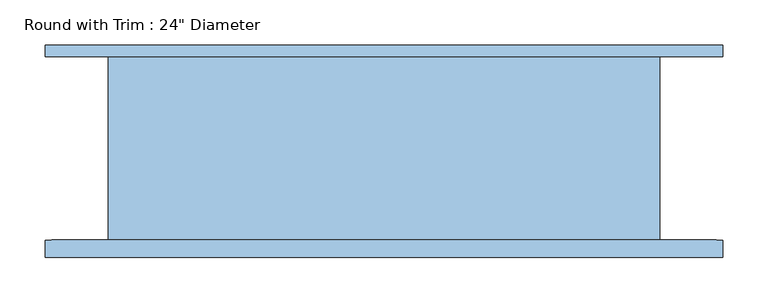
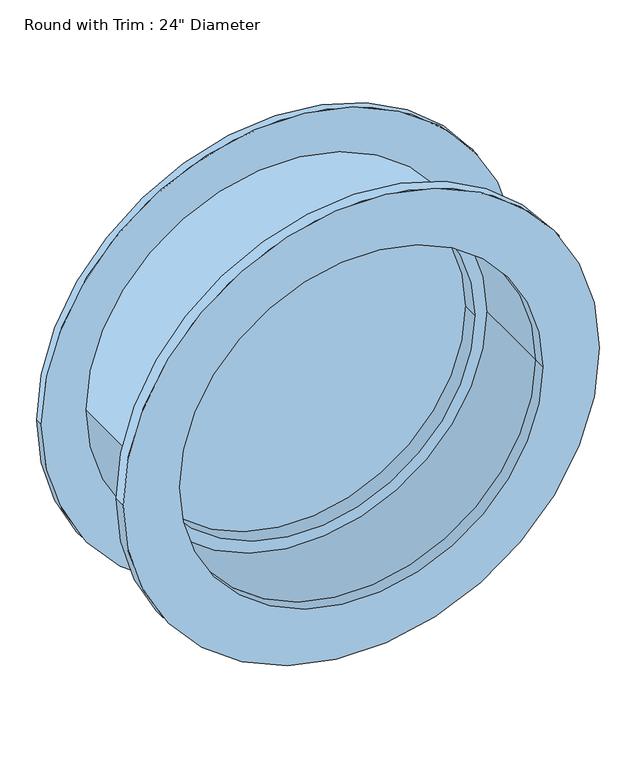
"""IFC4 building model written with IfcOpenShell, lengths in millimetres: window geometry."""

from ifc_helpers import new_model, si_unit, point, frame, frame_2d, origin, place, context, project, spatial, circle_curve, trimmed, segment, composite_curve, outline, extrude, source, transform, mapped, element, save


def window_99b8bbb7(model_context):
    return source(origin(), model_context, "Body", "SweptSolid", [
        extrude(outline(composite_curve([segment(trimmed(circle_curve(frame_2d((1219.2, -152.4)), 374.65), [point((1219.2, -527.05))], [point((1219.2, 222.25))], False, "CARTESIAN"), True, "CONTINUOUS"), segment(trimmed(circle_curve(frame_2d((1219.2, -152.4)), 374.65), [point((1219.2, 222.25))], [point((1219.2, -527.05))], False, "CARTESIAN"), True, "CONTINUOUS")], self_intersect=False), holes=[composite_curve([segment(trimmed(circle_curve(frame_2d((1219.2, -152.4)), 285.75), [point((1219.2, -438.15))], [point((1219.2, 133.35))], True, "CARTESIAN"), True, "CONTINUOUS"), segment(trimmed(circle_curve(frame_2d((1219.2, -152.4)), 285.75), [point((1219.2, 133.35))], [point((1219.2, -438.15))], True, "CARTESIAN"), True, "CONTINUOUS")], self_intersect=False)]), frame((0.0, -120.65, 0.0), z_axis=(0.0, 1.0, 0.0), x_axis=(0.0, 0.0, 1.0)), (0.0, 0.0, 1.0), 19.05),
        extrude(outline(composite_curve([segment(trimmed(circle_curve(frame_2d((1219.2, -152.4)), 374.65), [point((1219.2, -527.05))], [point((1219.2, 222.25))], False, "CARTESIAN"), True, "CONTINUOUS"), segment(trimmed(circle_curve(frame_2d((1219.2, -152.4)), 374.65), [point((1219.2, 222.25))], [point((1219.2, -527.05))], False, "CARTESIAN"), True, "CONTINUOUS")], self_intersect=False), holes=[composite_curve([segment(trimmed(circle_curve(frame_2d((1219.2, -152.4)), 285.75), [point((1219.2, -438.15))], [point((1219.2, 133.35))], True, "CARTESIAN"), True, "CONTINUOUS"), segment(trimmed(circle_curve(frame_2d((1219.2, -152.4)), 285.75), [point((1219.2, 133.35))], [point((1219.2, -438.15))], True, "CARTESIAN"), True, "CONTINUOUS")], self_intersect=False)]), frame((0.0, 101.6, 0.0), z_axis=(0.0, 1.0, 0.0), x_axis=(0.0, 0.0, 1.0)), (0.0, 0.0, 1.0), 12.7),
        extrude(outline(composite_curve([segment(trimmed(circle_curve(frame_2d((1219.2, -152.4)), 266.7), [point((1219.2, -419.1))], [point((1219.2, 114.3))], False, "CARTESIAN"), True, "CONTINUOUS"), segment(trimmed(circle_curve(frame_2d((1219.2, -152.4)), 266.7), [point((1219.2, 114.3))], [point((1219.2, -419.1))], False, "CARTESIAN"), True, "CONTINUOUS")], self_intersect=False)), frame((0.0, 57.15, 0.0), z_axis=(0.0, 1.0, 0.0), x_axis=(0.0, 0.0, 1.0)), (0.0, 0.0, 1.0), 12.7),
        extrude(outline(composite_curve([segment(trimmed(circle_curve(frame_2d((1219.2, -152.4)), 285.75), [point((1219.2, -438.15))], [point((1219.2, 133.35))], False, "CARTESIAN"), True, "CONTINUOUS"), segment(trimmed(circle_curve(frame_2d((1219.2, -152.4)), 285.75), [point((1219.2, 133.35))], [point((1219.2, -438.15))], False, "CARTESIAN"), True, "CONTINUOUS")], self_intersect=False), holes=[composite_curve([segment(trimmed(circle_curve(frame_2d((1219.2, -152.4)), 266.7), [point((1219.2, -419.1))], [point((1219.2, 114.3))], True, "CARTESIAN"), True, "CONTINUOUS"), segment(trimmed(circle_curve(frame_2d((1219.2, -152.4)), 266.7), [point((1219.2, 114.3))], [point((1219.2, -419.1))], True, "CARTESIAN"), True, "CONTINUOUS")], self_intersect=False)]), frame((0.0, 31.75, 0.0), z_axis=(0.0, 1.0, 0.0), x_axis=(0.0, 0.0, 1.0)), (0.0, 0.0, 1.0), 50.8),
        extrude(outline(composite_curve([segment(trimmed(circle_curve(frame_2d((1219.2, -152.4)), 304.8), [point((1219.2, -457.2))], [point((1219.2, 152.4))], False, "CARTESIAN"), True, "CONTINUOUS"), segment(trimmed(circle_curve(frame_2d((1219.2, -152.4)), 304.8), [point((1219.2, 152.4))], [point((1219.2, -457.2))], False, "CARTESIAN"), True, "CONTINUOUS")], self_intersect=False), holes=[composite_curve([segment(trimmed(circle_curve(frame_2d((1219.2, -152.4)), 285.75), [point((1219.2, -438.15))], [point((1219.2, 133.35))], True, "CARTESIAN"), True, "CONTINUOUS"), segment(trimmed(circle_curve(frame_2d((1219.2, -152.4)), 285.75), [point((1219.2, 133.35))], [point((1219.2, -438.15))], True, "CARTESIAN"), True, "CONTINUOUS")], self_intersect=False)]), frame((0.0, -101.6, 0.0), z_axis=(0.0, 1.0, 0.0), x_axis=(0.0, 0.0, 1.0)), (0.0, 0.0, 1.0), 203.2),
    ])


if __name__ == "__main__":
    model = new_model("IFC4")
    model_context = context("Model", 3, world=origin())
    ifc_project = project(units=[si_unit("LENGTHUNIT", "METRE", prefix="MILLI")], contexts=[model_context])
    site = spatial("IfcSite", under=ifc_project)
    building = spatial("IfcBuilding", under=site)
    placement = place(None, origin())
    window_shape = window_99b8bbb7(model_context)
    element("IfcWindow", 1, ObjectType="Round with Trim : 24\" Diameter", at=placement, inside=building, context=model_context, shape_type="MappedRepresentation", body=[
        mapped(window_shape, transform((0.0, 0.0, 0.0), x_axis=(1.0, 0.0, 0.0), y_axis=(0.0, 1.0, 0.0), z_axis=(0.0, 0.0, 1.0))),
    ])
    save(model, "model.ifc")

# Revit data of these elements
# Type "Round with Trim : 24\" Diameter"
#   Type Mark = "28"
#   Construction Type Id = "GSP4R"
#   Assembly Code = "B2020100"
#   Analytic Construction = "1/8 in Pilkington single glazing"
#   Visual Light Transmittance = 0.9
#   Solar Heat Gain Coefficient = 0.78
#   Heat Transfer Coefficient (U) = 0.6496 BTU/(h·ft²·°F)
#   Default Sill Height = 3' - 0"
#   Trim Projection - Ext. = 0' - 0 1/2"
#   Trim Projection - Int. = 0' - 0 3/4"
#   Trim Width - Exterior = 0' - 3 1/2"
#   Trim Width - Interior = 0' - 3 1/2"
#   Width = 2' - 0"
#   Define Thermal Properties by = 1
#   Glass Pane Material = Glass
#   Sash Material = Sash
#   Trim Exterior Material = Trim
#   Trim Interior Material = Trim
#   Wall Closure = (empty or 0)
# Element 1 (IfcWindow, "Round with Trim : 24\" Diameter")
#   Materials on its faces: "Trim", "Sash", "Glass"
# Materials
#   "Glass": class "Glass", colour RGB 0 128 192, transparency 0.75, Description = "Soda Lime Glass", Cost = 0
#   "Sash": class "Wood", colour RGB 224 178 126, transparency 0
#   "Trim": class "Wood", colour RGB 224 178 126, transparency 0
